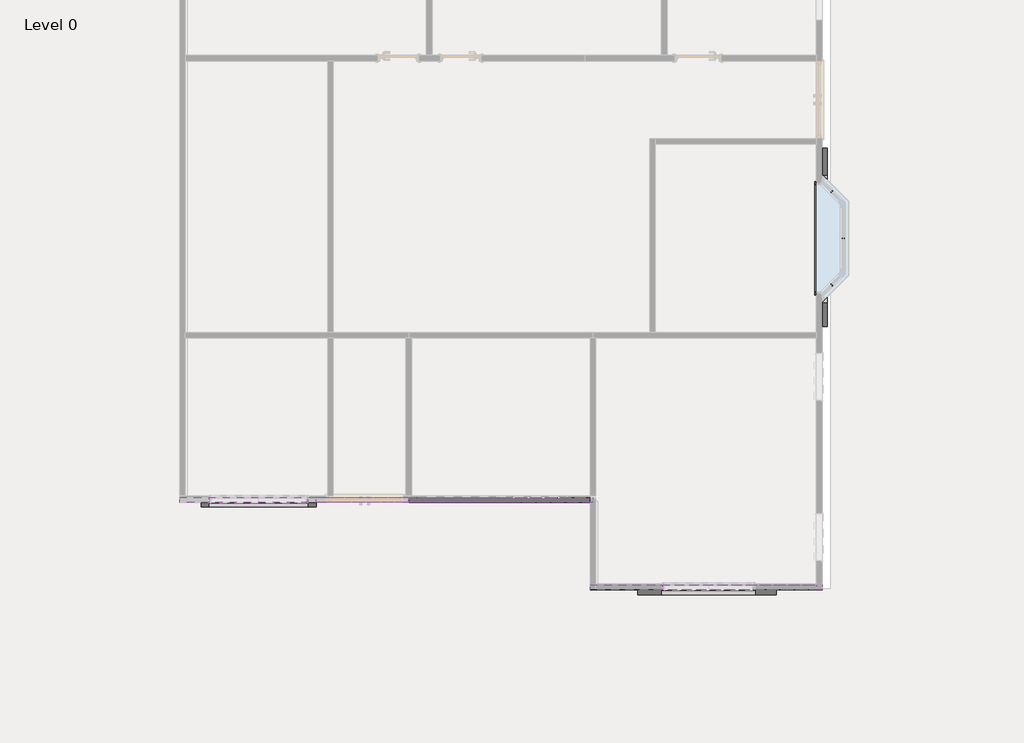
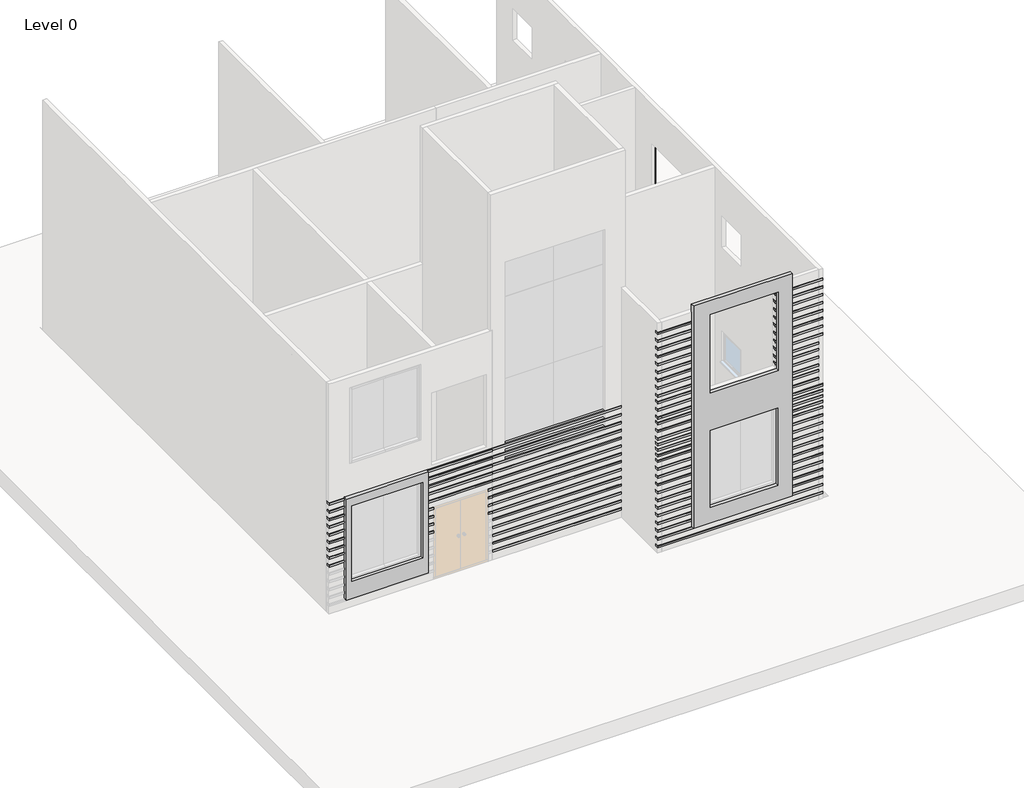
# One storey, part 5 of 5: 60 proxies.
"""IFC4 building model written with IfcOpenShell, lengths in millimetres."""

from ifc_helpers import new_model, si_unit, frame, origin, place, context, project, spatial, polyline, outline, extrude, transform, mapped, element, save
from components import generic_models_1_generic_models_1_954afae2, generic_models_4_generic_models_4_8888209d, generic_models_7_generic_models_7_fc47f9bb, muntin_pattern_2x2_muntin_pattern_2x2_511ed329, muntin_pattern_2x2_muntin_pattern_2x2_63bd3b25, trim_window_interior_flat_picture_frame_e25f2530

model = new_model("IFC4")

# Units and contexts
model_context = context("Model", 3, world=origin())
ifc_project = project(units=[si_unit("LENGTHUNIT", "METRE", prefix="MILLI")], contexts=[model_context])

# Site, building, storey
site = spatial("IfcSite", under=ifc_project)
building = spatial("IfcBuilding", under=site)
storey = spatial("IfcBuildingStorey", under=building, Name="Level 0", Elevation=0.0)

# Proxies
placement = place(None, origin())
element("IfcBuildingElementProxy", 1, Name="Cornice", ObjectType="Cornice", at=placement, inside=storey, context=model_context, shape_type="SweptSolid", body=[
    extrude(outline(polyline([(-2780.5468048, 1828.8), (-2883.0468048, 1828.8), (-2883.0468048, 1883.8), (-2863.0468048, 1903.8), (-2780.5468048, 1903.8), (-2780.5468048, 1828.8)])), frame((-14910.579089, 0.0, 0.0), z_axis=(1.0, 0.0, 0.0), x_axis=(0.0, 1.0, 0.0)), (0.0, 0.0, 1.0), 3562.35),
])
element("IfcBuildingElementProxy", 2, Name="Cornice", ObjectType="Cornice", at=placement, inside=storey, context=model_context, shape_type="SweptSolid", body=[
    extrude(outline(polyline([(-2780.5468048, 2057.4), (-2883.0468048, 2057.4), (-2883.0468048, 2112.4), (-2863.0468048, 2132.4), (-2780.5468048, 2132.4), (-2780.5468048, 2057.4)])), frame((-14910.579089, 0.0, 0.0), z_axis=(1.0, 0.0, 0.0), x_axis=(0.0, 1.0, 0.0)), (0.0, 0.0, 1.0), 3562.35),
])
element("IfcBuildingElementProxy", 3, Name="Cornice", ObjectType="Cornice", at=placement, inside=storey, context=model_context, shape_type="SweptSolid", body=[
    extrude(outline(polyline([(-2780.5468048, 2286.0), (-2883.0468048, 2286.0), (-2883.0468048, 2341.0), (-2863.0468048, 2361.0), (-2780.5468048, 2361.0), (-2780.5468048, 2286.0)])), frame((-16727.530247, 0.0, 0.0), z_axis=(1.0, 0.0, 0.0), x_axis=(0.0, 1.0, 0.0)), (0.0, 0.0, 1.0), 5379.301158),
])
element("IfcBuildingElementProxy", 4, Name="Cornice", ObjectType="Cornice", at=placement, inside=storey, context=model_context, shape_type="SweptSolid", body=[
    extrude(outline(polyline([(-2780.5468048, 2514.6), (-2883.0468048, 2514.6), (-2883.0468048, 2569.6), (-2863.0468048, 2589.6), (-2780.5468048, 2589.6), (-2780.5468048, 2514.6)])), frame((-16727.530247, 0.0, 0.0), z_axis=(1.0, 0.0, 0.0), x_axis=(0.0, 1.0, 0.0)), (0.0, 0.0, 1.0), 5379.301158),
])
element("IfcBuildingElementProxy", 5, Name="Cornice", ObjectType="Cornice", at=placement, inside=storey, context=model_context, shape_type="SweptSolid", body=[
    extrude(outline(polyline([(-2780.5468048, 1600.2), (-2883.0468048, 1600.2), (-2883.0468048, 1655.2), (-2863.0468048, 1675.2), (-2780.5468048, 1675.2), (-2780.5468048, 1600.2)])), frame((-14910.579089, 0.0, 0.0), z_axis=(1.0, 0.0, 0.0), x_axis=(0.0, 1.0, 0.0)), (0.0, 0.0, 1.0), 3562.35),
])
element("IfcBuildingElementProxy", 6, Name="Cornice", ObjectType="Cornice", at=placement, inside=storey, context=model_context, shape_type="SweptSolid", body=[
    extrude(outline(polyline([(-2780.5468048, 1371.6), (-2883.0468048, 1371.6), (-2883.0468048, 1426.6), (-2863.0468048, 1446.6), (-2780.5468048, 1446.6), (-2780.5468048, 1371.6)])), frame((-14910.579089, 0.0, 0.0), z_axis=(1.0, 0.0, 0.0), x_axis=(0.0, 1.0, 0.0)), (0.0, 0.0, 1.0), 3562.35),
])
element("IfcBuildingElementProxy", 7, Name="Cornice", ObjectType="Cornice", at=placement, inside=storey, context=model_context, shape_type="SweptSolid", body=[
    extrude(outline(polyline([(-2780.5468048, 1143.0), (-2883.0468048, 1143.0), (-2883.0468048, 1198.0), (-2863.0468048, 1218.0), (-2780.5468048, 1218.0), (-2780.5468048, 1143.0)])), frame((-14910.579089, 0.0, 0.0), z_axis=(1.0, 0.0, 0.0), x_axis=(0.0, 1.0, 0.0)), (0.0, 0.0, 1.0), 3562.35),
])
element("IfcBuildingElementProxy", 8, Name="Cornice", ObjectType="Cornice", at=placement, inside=storey, context=model_context, shape_type="SweptSolid", body=[
    extrude(outline(polyline([(-2780.5468048, 914.4), (-2883.0468048, 914.4), (-2883.0468048, 969.4), (-2863.0468048, 989.4), (-2780.5468048, 989.4), (-2780.5468048, 914.4)])), frame((-14910.579089, 0.0, 0.0), z_axis=(1.0, 0.0, 0.0), x_axis=(0.0, 1.0, 0.0)), (0.0, 0.0, 1.0), 3562.35),
])
element("IfcBuildingElementProxy", 9, Name="Cornice", ObjectType="Cornice", at=placement, inside=storey, context=model_context, shape_type="SweptSolid", body=[
    extrude(outline(polyline([(-2780.5468048, 685.8), (-2883.0468048, 685.8), (-2883.0468048, 740.8), (-2863.0468048, 760.8), (-2780.5468048, 760.8), (-2780.5468048, 685.8)])), frame((-14910.579089, 0.0, 0.0), z_axis=(1.0, 0.0, 0.0), x_axis=(0.0, 1.0, 0.0)), (0.0, 0.0, 1.0), 3562.35),
])
element("IfcBuildingElementProxy", 10, Name="Cornice", ObjectType="Cornice", at=placement, inside=storey, context=model_context, shape_type="SweptSolid", body=[
    extrude(outline(polyline([(-2780.5468048, 457.2), (-2883.0468048, 457.2), (-2883.0468048, 512.2), (-2863.0468048, 532.2), (-2780.5468048, 532.2), (-2780.5468048, 457.2)])), frame((-14910.579089, 0.0, 0.0), z_axis=(1.0, 0.0, 0.0), x_axis=(0.0, 1.0, 0.0)), (0.0, 0.0, 1.0), 3562.35),
])
element("IfcBuildingElementProxy", 11, Name="Cornice", ObjectType="Cornice", at=placement, inside=storey, context=model_context, shape_type="SweptSolid", body=[
    extrude(outline(polyline([(-2780.5468048, 228.6), (-2883.0468048, 228.6), (-2883.0468048, 283.6), (-2863.0468048, 303.6), (-2780.5468048, 303.6), (-2780.5468048, 228.6)])), frame((-14910.579089, 0.0, 0.0), z_axis=(1.0, 0.0, 0.0), x_axis=(0.0, 1.0, 0.0)), (0.0, 0.0, 1.0), 3562.35),
])
element("IfcBuildingElementProxy", 12, Name="Cornice", ObjectType="Cornice", at=placement, inside=storey, context=model_context, shape_type="SweptSolid", body=[
    extrude(outline(polyline([(-2780.5468048, 2743.2), (-2883.0468048, 2743.2), (-2883.0468048, 2798.2), (-2863.0468048, 2818.2), (-2780.5468048, 2818.2), (-2780.5468048, 2743.2)])), frame((-16727.530247, 0.0, 0.0), z_axis=(1.0, 0.0, 0.0), x_axis=(0.0, 1.0, 0.0)), (0.0, 0.0, 1.0), 5436.451158),
    extrude(outline(polyline([(-2780.5468048, 2743.2), (-2883.0468048, 2743.2), (-2883.0468048, 2798.2), (-2863.0468048, 2818.2), (-2780.5468048, 2818.2), (-2780.5468048, 2743.2)])), frame((-16727.530247, 0.0, 0.0), z_axis=(1.0, 0.0, 0.0), x_axis=(0.0, 1.0, 0.0)), (0.0, 0.0, 1.0), 5436.451158),
])
element("IfcBuildingElementProxy", 13, Name="Cornice", ObjectType="Cornice", at=placement, inside=storey, context=model_context, shape_type="SweptSolid", body=[
    extrude(outline(polyline([(-2780.5468048, 2971.8), (-2883.0468048, 2971.8), (-2883.0468048, 3026.8), (-2863.0468048, 3046.8), (-2780.5468048, 3046.8), (-2780.5468048, 2971.8)])), frame((-16727.530247, 0.0, 0.0), z_axis=(1.0, 0.0, 0.0), x_axis=(0.0, 1.0, 0.0)), (0.0, 0.0, 1.0), 5436.451158),
    extrude(outline(polyline([(-2780.5468048, 2971.8), (-2883.0468048, 2971.8), (-2883.0468048, 3026.8), (-2863.0468048, 3046.8), (-2780.5468048, 3046.8), (-2780.5468048, 2971.8)])), frame((-16727.530247, 0.0, 0.0), z_axis=(1.0, 0.0, 0.0), x_axis=(0.0, 1.0, 0.0)), (0.0, 0.0, 1.0), 5436.451158),
])
element("IfcBuildingElementProxy", 14, Name="Cornice", ObjectType="Cornice", at=placement, inside=storey, context=model_context, shape_type="SweptSolid", body=[
    extrude(outline(polyline([(-2780.5468048, 3200.4), (-2883.0468048, 3200.4), (-2883.0468048, 3255.4), (-2863.0468048, 3275.4), (-2780.5468048, 3275.4), (-2780.5468048, 3200.4)])), frame((-16727.530247, 0.0, 0.0), z_axis=(1.0, 0.0, 0.0), x_axis=(0.0, 1.0, 0.0)), (0.0, 0.0, 1.0), 5436.451158),
    extrude(outline(polyline([(-2780.5468048, 3200.4), (-2883.0468048, 3200.4), (-2883.0468048, 3255.4), (-2863.0468048, 3275.4), (-2780.5468048, 3275.4), (-2780.5468048, 3200.4)])), frame((-16727.530247, 0.0, 0.0), z_axis=(1.0, 0.0, 0.0), x_axis=(0.0, 1.0, 0.0)), (0.0, 0.0, 1.0), 5436.451158),
])
element("IfcBuildingElementProxy", 15, Name="Cornice", ObjectType="Cornice", at=placement, inside=storey, context=model_context, shape_type="SweptSolid", body=[
    extrude(outline(polyline([(-4501.3968048, 152.4), (-4603.8968048, 152.4), (-4603.8968048, 207.4), (-4583.8968048, 227.4), (-4501.3968048, 227.4), (-4501.3968048, 152.4)])), frame((-11348.229089, 0.0, 0.0), z_axis=(1.0, 0.0, 0.0), x_axis=(0.0, 1.0, 0.0)), (0.0, 0.0, 1.0), 4559.3),
])
element("IfcBuildingElementProxy", 16, Name="Cornice", ObjectType="Cornice", at=placement, inside=storey, context=model_context, shape_type="SweptSolid", body=[
    extrude(outline(polyline([(-4501.3968048, 381.0), (-4603.8968048, 381.0), (-4603.8968048, 436.0), (-4583.8968048, 456.0), (-4501.3968048, 456.0), (-4501.3968048, 381.0)])), frame((-11348.229089, 0.0, 0.0), z_axis=(1.0, 0.0, 0.0), x_axis=(0.0, 1.0, 0.0)), (0.0, 0.0, 1.0), 4559.3),
])
element("IfcBuildingElementProxy", 17, Name="Cornice", ObjectType="Cornice", at=placement, inside=storey, context=model_context, shape_type="SweptSolid", body=[
    extrude(outline(polyline([(-4501.3968048, 609.6), (-4603.8968048, 609.6), (-4603.8968048, 664.6), (-4583.8968048, 684.6), (-4501.3968048, 684.6), (-4501.3968048, 609.6)])), frame((-11348.229089, 0.0, 0.0), z_axis=(1.0, 0.0, 0.0), x_axis=(0.0, 1.0, 0.0)), (0.0, 0.0, 1.0), 4559.3),
])
element("IfcBuildingElementProxy", 18, Name="Cornice", ObjectType="Cornice", at=placement, inside=storey, context=model_context, shape_type="SweptSolid", body=[
    extrude(outline(polyline([(-4501.3968048, 830.4106439), (-4603.8968048, 830.4106439), (-4603.8968048, 885.4106439), (-4583.8968048, 905.4106439), (-4501.3968048, 905.4106439), (-4501.3968048, 830.4106439)])), frame((-11348.229089, 0.0, 0.0), z_axis=(1.0, 0.0, 0.0), x_axis=(0.0, 1.0, 0.0)), (0.0, 0.0, 1.0), 4559.3),
])
element("IfcBuildingElementProxy", 19, Name="Cornice", ObjectType="Cornice", at=placement, inside=storey, context=model_context, shape_type="SweptSolid", body=[
    extrude(outline(polyline([(-4501.3968048, 1059.0106439), (-4603.8968048, 1059.0106439), (-4603.8968048, 1114.0106439), (-4583.8968048, 1134.0106439), (-4501.3968048, 1134.0106439), (-4501.3968048, 1059.0106439)])), frame((-8102.129089, 0.0, 0.0), z_axis=(1.0, 0.0, 0.0), x_axis=(0.0, 1.0, 0.0)), (0.0, 0.0, 1.0), 1313.2),
    extrude(outline(polyline([(-4501.3968048, 1059.0106439), (-4603.8968048, 1059.0106439), (-4603.8968048, 1114.0106439), (-4583.8968048, 1134.0106439), (-4501.3968048, 1134.0106439), (-4501.3968048, 1059.0106439)])), frame((-11348.229089, 0.0, 0.0), z_axis=(1.0, 0.0, 0.0), x_axis=(0.0, 1.0, 0.0)), (0.0, 0.0, 1.0), 1417.3),
])
element("IfcBuildingElementProxy", 20, Name="Cornice", ObjectType="Cornice", at=placement, inside=storey, context=model_context, shape_type="SweptSolid", body=[
    extrude(outline(polyline([(-4501.3968048, 1279.8212878), (-4603.8968048, 1279.8212878), (-4603.8968048, 1334.8212878), (-4583.8968048, 1354.8212878), (-4501.3968048, 1354.8212878), (-4501.3968048, 1279.8212878)])), frame((-8102.129089, 0.0, 0.0), z_axis=(1.0, 0.0, 0.0), x_axis=(0.0, 1.0, 0.0)), (0.0, 0.0, 1.0), 1313.2),
    extrude(outline(polyline([(-4501.3968048, 1279.8212878), (-4603.8968048, 1279.8212878), (-4603.8968048, 1334.8212878), (-4583.8968048, 1354.8212878), (-4501.3968048, 1354.8212878), (-4501.3968048, 1279.8212878)])), frame((-11348.229089, 0.0, 0.0), z_axis=(1.0, 0.0, 0.0), x_axis=(0.0, 1.0, 0.0)), (0.0, 0.0, 1.0), 1417.3),
])
element("IfcBuildingElementProxy", 21, Name="Cornice", ObjectType="Cornice", at=placement, inside=storey, context=model_context, shape_type="SweptSolid", body=[
    extrude(outline(polyline([(-4501.3968048, 1500.6319317), (-4603.8968048, 1500.6319317), (-4603.8968048, 1555.6319317), (-4583.8968048, 1575.6319317), (-4501.3968048, 1575.6319317), (-4501.3968048, 1500.6319317)])), frame((-8102.129089, 0.0, 0.0), z_axis=(1.0, 0.0, 0.0), x_axis=(0.0, 1.0, 0.0)), (0.0, 0.0, 1.0), 1313.2),
    extrude(outline(polyline([(-4501.3968048, 1500.6319317), (-4603.8968048, 1500.6319317), (-4603.8968048, 1555.6319317), (-4583.8968048, 1575.6319317), (-4501.3968048, 1575.6319317), (-4501.3968048, 1500.6319317)])), frame((-11348.229089, 0.0, 0.0), z_axis=(1.0, 0.0, 0.0), x_axis=(0.0, 1.0, 0.0)), (0.0, 0.0, 1.0), 1417.3),
])
element("IfcBuildingElementProxy", 22, Name="Cornice", ObjectType="Cornice", at=placement, inside=storey, context=model_context, shape_type="SweptSolid", body=[
    extrude(outline(polyline([(-4501.3968048, 1729.2319317), (-4603.8968048, 1729.2319317), (-4603.8968048, 1784.2319317), (-4583.8968048, 1804.2319317), (-4501.3968048, 1804.2319317), (-4501.3968048, 1729.2319317)])), frame((-8102.129089, 0.0, 0.0), z_axis=(1.0, 0.0, 0.0), x_axis=(0.0, 1.0, 0.0)), (0.0, 0.0, 1.0), 1313.2),
    extrude(outline(polyline([(-4501.3968048, 1729.2319317), (-4603.8968048, 1729.2319317), (-4603.8968048, 1784.2319317), (-4583.8968048, 1804.2319317), (-4501.3968048, 1804.2319317), (-4501.3968048, 1729.2319317)])), frame((-11348.229089, 0.0, 0.0), z_axis=(1.0, 0.0, 0.0), x_axis=(0.0, 1.0, 0.0)), (0.0, 0.0, 1.0), 1417.3),
])
element("IfcBuildingElementProxy", 23, Name="Cornice", ObjectType="Cornice", at=placement, inside=storey, context=model_context, shape_type="SweptSolid", body=[
    extrude(outline(polyline([(-4501.3968048, 1957.8319317), (-4603.8968048, 1957.8319317), (-4603.8968048, 2012.8319317), (-4583.8968048, 2032.8319317), (-4501.3968048, 2032.8319317), (-4501.3968048, 1957.8319317)])), frame((-8102.129089, 0.0, 0.0), z_axis=(1.0, 0.0, 0.0), x_axis=(0.0, 1.0, 0.0)), (0.0, 0.0, 1.0), 1313.2),
    extrude(outline(polyline([(-4501.3968048, 1957.8319317), (-4603.8968048, 1957.8319317), (-4603.8968048, 2012.8319317), (-4583.8968048, 2032.8319317), (-4501.3968048, 2032.8319317), (-4501.3968048, 1957.8319317)])), frame((-11348.229089, 0.0, 0.0), z_axis=(1.0, 0.0, 0.0), x_axis=(0.0, 1.0, 0.0)), (0.0, 0.0, 1.0), 1417.3),
])
element("IfcBuildingElementProxy", 24, Name="Cornice", ObjectType="Cornice", at=placement, inside=storey, context=model_context, shape_type="SweptSolid", body=[
    extrude(outline(polyline([(-4501.3968048, 2186.4319317), (-4603.8968048, 2186.4319317), (-4603.8968048, 2241.4319317), (-4583.8968048, 2261.4319317), (-4501.3968048, 2261.4319317), (-4501.3968048, 2186.4319317)])), frame((-8102.129089, 0.0, 0.0), z_axis=(1.0, 0.0, 0.0), x_axis=(0.0, 1.0, 0.0)), (0.0, 0.0, 1.0), 1313.2),
    extrude(outline(polyline([(-4501.3968048, 2186.4319317), (-4603.8968048, 2186.4319317), (-4603.8968048, 2241.4319317), (-4583.8968048, 2261.4319317), (-4501.3968048, 2261.4319317), (-4501.3968048, 2186.4319317)])), frame((-11348.229089, 0.0, 0.0), z_axis=(1.0, 0.0, 0.0), x_axis=(0.0, 1.0, 0.0)), (0.0, 0.0, 1.0), 1417.3),
])
element("IfcBuildingElementProxy", 25, Name="Cornice", ObjectType="Cornice", at=placement, inside=storey, context=model_context, shape_type="SweptSolid", body=[
    extrude(outline(polyline([(-4501.3968048, 2415.0319317), (-4603.8968048, 2415.0319317), (-4603.8968048, 2470.0319317), (-4583.8968048, 2490.0319317), (-4501.3968048, 2490.0319317), (-4501.3968048, 2415.0319317)])), frame((-8102.129089, 0.0, 0.0), z_axis=(1.0, 0.0, 0.0), x_axis=(0.0, 1.0, 0.0)), (0.0, 0.0, 1.0), 1313.2),
    extrude(outline(polyline([(-4501.3968048, 2415.0319317), (-4603.8968048, 2415.0319317), (-4603.8968048, 2470.0319317), (-4583.8968048, 2490.0319317), (-4501.3968048, 2490.0319317), (-4501.3968048, 2415.0319317)])), frame((-11348.229089, 0.0, 0.0), z_axis=(1.0, 0.0, 0.0), x_axis=(0.0, 1.0, 0.0)), (0.0, 0.0, 1.0), 1417.3),
])
element("IfcBuildingElementProxy", 26, Name="Cornice", ObjectType="Cornice", at=placement, inside=storey, context=model_context, shape_type="SweptSolid", body=[
    extrude(outline(polyline([(-4501.3968048, 2643.6319317), (-4603.8968048, 2643.6319317), (-4603.8968048, 2698.6319317), (-4583.8968048, 2718.6319317), (-4501.3968048, 2718.6319317), (-4501.3968048, 2643.6319317)])), frame((-8102.129089, 0.0, 0.0), z_axis=(1.0, 0.0, 0.0), x_axis=(0.0, 1.0, 0.0)), (0.0, 0.0, 1.0), 1313.2),
    extrude(outline(polyline([(-4501.3968048, 2643.6319317), (-4603.8968048, 2643.6319317), (-4603.8968048, 2698.6319317), (-4583.8968048, 2718.6319317), (-4501.3968048, 2718.6319317), (-4501.3968048, 2643.6319317)])), frame((-11348.229089, 0.0, 0.0), z_axis=(1.0, 0.0, 0.0), x_axis=(0.0, 1.0, 0.0)), (0.0, 0.0, 1.0), 1417.3),
])
element("IfcBuildingElementProxy", 27, Name="Cornice", ObjectType="Cornice", at=placement, inside=storey, context=model_context, shape_type="SweptSolid", body=[
    extrude(outline(polyline([(-4501.3968048, 2805.2765418), (-4603.8968048, 2805.2765418), (-4603.8968048, 2860.2765418), (-4583.8968048, 2880.2765418), (-4501.3968048, 2880.2765418), (-4501.3968048, 2805.2765418)])), frame((-8102.129089, 0.0, 0.0), z_axis=(1.0, 0.0, 0.0), x_axis=(0.0, 1.0, 0.0)), (0.0, 0.0, 1.0), 1313.2),
    extrude(outline(polyline([(-4501.3968048, 2805.2765418), (-4603.8968048, 2805.2765418), (-4603.8968048, 2860.2765418), (-4583.8968048, 2880.2765418), (-4501.3968048, 2880.2765418), (-4501.3968048, 2805.2765418)])), frame((-11348.229089, 0.0, 0.0), z_axis=(1.0, 0.0, 0.0), x_axis=(0.0, 1.0, 0.0)), (0.0, 0.0, 1.0), 1417.3),
])
element("IfcBuildingElementProxy", 28, Name="Cornice", ObjectType="Cornice", at=placement, inside=storey, context=model_context, shape_type="SweptSolid", body=[
    extrude(outline(polyline([(-4501.3968048, 2966.921152), (-4603.8968048, 2966.921152), (-4603.8968048, 3021.921152), (-4583.8968048, 3041.921152), (-4501.3968048, 3041.921152), (-4501.3968048, 2966.921152)])), frame((-8102.129089, 0.0, 0.0), z_axis=(1.0, 0.0, 0.0), x_axis=(0.0, 1.0, 0.0)), (0.0, 0.0, 1.0), 1313.2),
    extrude(outline(polyline([(-4501.3968048, 2966.921152), (-4603.8968048, 2966.921152), (-4603.8968048, 3021.921152), (-4583.8968048, 3041.921152), (-4501.3968048, 3041.921152), (-4501.3968048, 2966.921152)])), frame((-11348.229089, 0.0, 0.0), z_axis=(1.0, 0.0, 0.0), x_axis=(0.0, 1.0, 0.0)), (0.0, 0.0, 1.0), 1417.3),
])
element("IfcBuildingElementProxy", 29, Name="Cornice", ObjectType="Cornice", at=placement, inside=storey, context=model_context, shape_type="SweptSolid", body=[
    extrude(outline(polyline([(-4501.3968048, 3128.5657622), (-4603.8968048, 3128.5657622), (-4603.8968048, 3183.5657622), (-4583.8968048, 3203.5657622), (-4501.3968048, 3203.5657622), (-4501.3968048, 3128.5657622)])), frame((-8102.129089, 0.0, 0.0), z_axis=(1.0, 0.0, 0.0), x_axis=(0.0, 1.0, 0.0)), (0.0, 0.0, 1.0), 1313.2),
    extrude(outline(polyline([(-4501.3968048, 3128.5657622), (-4603.8968048, 3128.5657622), (-4603.8968048, 3183.5657622), (-4583.8968048, 3203.5657622), (-4501.3968048, 3203.5657622), (-4501.3968048, 3128.5657622)])), frame((-11348.229089, 0.0, 0.0), z_axis=(1.0, 0.0, 0.0), x_axis=(0.0, 1.0, 0.0)), (0.0, 0.0, 1.0), 1417.3),
])
element("IfcBuildingElementProxy", 30, Name="Cornice", ObjectType="Cornice", at=placement, inside=storey, context=model_context, shape_type="SweptSolid", body=[
    extrude(outline(polyline([(-2780.5468048, 1371.6), (-2883.0468048, 1371.6), (-2883.0468048, 1426.6), (-2863.0468048, 1446.6), (-2780.5468048, 1446.6), (-2780.5468048, 1371.6)])), frame((-15018.529089, 0.0, 0.0), z_axis=(1.0, 0.0, 0.0), x_axis=(0.0, 1.0, 0.0)), (0.0, 0.0, 1.0), 107.95),
    extrude(outline(polyline([(-2780.5468048, 1371.6), (-2883.0468048, 1371.6), (-2883.0468048, 1426.6), (-2863.0468048, 1446.6), (-2780.5468048, 1446.6), (-2780.5468048, 1371.6)])), frame((-16885.429089, 0.0, 0.0), z_axis=(1.0, 0.0, 0.0), x_axis=(0.0, 1.0, 0.0)), (0.0, 0.0, 1.0), 356.9),
    extrude(outline(polyline([(-2780.5468048, 1371.6), (-2883.0468048, 1371.6), (-2883.0468048, 1426.6), (-2863.0468048, 1446.6), (-2780.5468048, 1446.6), (-2780.5468048, 1371.6)])), frame((-19412.729089, 0.0, 0.0), z_axis=(1.0, 0.0, 0.0), x_axis=(0.0, 1.0, 0.0)), (0.0, 0.0, 1.0), 571.5),
])
element("IfcBuildingElementProxy", 31, Name="Cornice", ObjectType="Cornice", at=placement, inside=storey, context=model_context, shape_type="SweptSolid", body=[
    extrude(outline(polyline([(-2780.5468048, 1600.2), (-2883.0468048, 1600.2), (-2883.0468048, 1655.2), (-2863.0468048, 1675.2), (-2780.5468048, 1675.2), (-2780.5468048, 1600.2)])), frame((-15018.529089, 0.0, 0.0), z_axis=(1.0, 0.0, 0.0), x_axis=(0.0, 1.0, 0.0)), (0.0, 0.0, 1.0), 107.95),
    extrude(outline(polyline([(-2780.5468048, 1600.2), (-2883.0468048, 1600.2), (-2883.0468048, 1655.2), (-2863.0468048, 1675.2), (-2780.5468048, 1675.2), (-2780.5468048, 1600.2)])), frame((-16885.429089, 0.0, 0.0), z_axis=(1.0, 0.0, 0.0), x_axis=(0.0, 1.0, 0.0)), (0.0, 0.0, 1.0), 356.9),
    extrude(outline(polyline([(-2780.5468048, 1600.2), (-2883.0468048, 1600.2), (-2883.0468048, 1655.2), (-2863.0468048, 1675.2), (-2780.5468048, 1675.2), (-2780.5468048, 1600.2)])), frame((-19412.729089, 0.0, 0.0), z_axis=(1.0, 0.0, 0.0), x_axis=(0.0, 1.0, 0.0)), (0.0, 0.0, 1.0), 571.5),
])
element("IfcBuildingElementProxy", 32, Name="Cornice", ObjectType="Cornice", at=placement, inside=storey, context=model_context, shape_type="SweptSolid", body=[
    extrude(outline(polyline([(-2780.5468048, 1821.0106439), (-2883.0468048, 1821.0106439), (-2883.0468048, 1876.0106439), (-2863.0468048, 1896.0106439), (-2780.5468048, 1896.0106439), (-2780.5468048, 1821.0106439)])), frame((-15018.529089, 0.0, 0.0), z_axis=(1.0, 0.0, 0.0), x_axis=(0.0, 1.0, 0.0)), (0.0, 0.0, 1.0), 107.95),
    extrude(outline(polyline([(-2780.5468048, 1821.0106439), (-2883.0468048, 1821.0106439), (-2883.0468048, 1876.0106439), (-2863.0468048, 1896.0106439), (-2780.5468048, 1896.0106439), (-2780.5468048, 1821.0106439)])), frame((-16885.429089, 0.0, 0.0), z_axis=(1.0, 0.0, 0.0), x_axis=(0.0, 1.0, 0.0)), (0.0, 0.0, 1.0), 356.9),
    extrude(outline(polyline([(-2780.5468048, 1821.0106439), (-2883.0468048, 1821.0106439), (-2883.0468048, 1876.0106439), (-2863.0468048, 1896.0106439), (-2780.5468048, 1896.0106439), (-2780.5468048, 1821.0106439)])), frame((-19412.729089, 0.0, 0.0), z_axis=(1.0, 0.0, 0.0), x_axis=(0.0, 1.0, 0.0)), (0.0, 0.0, 1.0), 571.5),
])
element("IfcBuildingElementProxy", 33, Name="Cornice", ObjectType="Cornice", at=placement, inside=storey, context=model_context, shape_type="SweptSolid", body=[
    extrude(outline(polyline([(-2780.5468048, 2049.6106439), (-2883.0468048, 2049.6106439), (-2883.0468048, 2104.6106439), (-2863.0468048, 2124.6106439), (-2780.5468048, 2124.6106439), (-2780.5468048, 2049.6106439)])), frame((-15018.529089, 0.0, 0.0), z_axis=(1.0, 0.0, 0.0), x_axis=(0.0, 1.0, 0.0)), (0.0, 0.0, 1.0), 107.95),
    extrude(outline(polyline([(-2780.5468048, 2049.6106439), (-2883.0468048, 2049.6106439), (-2883.0468048, 2104.6106439), (-2863.0468048, 2124.6106439), (-2780.5468048, 2124.6106439), (-2780.5468048, 2049.6106439)])), frame((-16885.429089, 0.0, 0.0), z_axis=(1.0, 0.0, 0.0), x_axis=(0.0, 1.0, 0.0)), (0.0, 0.0, 1.0), 356.9),
    extrude(outline(polyline([(-2780.5468048, 2049.6106439), (-2883.0468048, 2049.6106439), (-2883.0468048, 2104.6106439), (-2863.0468048, 2124.6106439), (-2780.5468048, 2124.6106439), (-2780.5468048, 2049.6106439)])), frame((-19412.729089, 0.0, 0.0), z_axis=(1.0, 0.0, 0.0), x_axis=(0.0, 1.0, 0.0)), (0.0, 0.0, 1.0), 571.5),
])
element("IfcBuildingElementProxy", 34, Name="Cornice", ObjectType="Cornice", at=placement, inside=storey, context=model_context, shape_type="SweptSolid", body=[
    extrude(outline(polyline([(-2780.5468048, 2278.2106439), (-2883.0468048, 2278.2106439), (-2883.0468048, 2333.2106439), (-2863.0468048, 2353.2106439), (-2780.5468048, 2353.2106439), (-2780.5468048, 2278.2106439)])), frame((-16885.429089, 0.0, 0.0), z_axis=(1.0, 0.0, 0.0), x_axis=(0.0, 1.0, 0.0)), (0.0, 0.0, 1.0), 1974.85),
    extrude(outline(polyline([(-2780.5468048, 2278.2106439), (-2883.0468048, 2278.2106439), (-2883.0468048, 2333.2106439), (-2863.0468048, 2353.2106439), (-2780.5468048, 2353.2106439), (-2780.5468048, 2278.2106439)])), frame((-19412.729089, 0.0, 0.0), z_axis=(1.0, 0.0, 0.0), x_axis=(0.0, 1.0, 0.0)), (0.0, 0.0, 1.0), 571.5),
])
element("IfcBuildingElementProxy", 35, Name="Cornice", ObjectType="Cornice", at=placement, inside=storey, context=model_context, shape_type="SweptSolid", body=[
    extrude(outline(polyline([(-2780.5468048, 2506.8106439), (-2883.0468048, 2506.8106439), (-2883.0468048, 2561.8106439), (-2863.0468048, 2581.8106439), (-2780.5468048, 2581.8106439), (-2780.5468048, 2506.8106439)])), frame((-16885.429089, 0.0, 0.0), z_axis=(1.0, 0.0, 0.0), x_axis=(0.0, 1.0, 0.0)), (0.0, 0.0, 1.0), 1974.85),
    extrude(outline(polyline([(-2780.5468048, 2506.8106439), (-2883.0468048, 2506.8106439), (-2883.0468048, 2561.8106439), (-2863.0468048, 2581.8106439), (-2780.5468048, 2581.8106439), (-2780.5468048, 2506.8106439)])), frame((-19412.729089, 0.0, 0.0), z_axis=(1.0, 0.0, 0.0), x_axis=(0.0, 1.0, 0.0)), (0.0, 0.0, 1.0), 571.5),
])
element("IfcBuildingElementProxy", 36, Name="Cornice", ObjectType="Cornice", at=placement, inside=storey, context=model_context, shape_type="SweptSolid", body=[
    extrude(outline(polyline([(-2780.5468048, 2720.4284072), (-2883.0468048, 2720.4284072), (-2883.0468048, 2775.4284072), (-2863.0468048, 2795.4284072), (-2780.5468048, 2795.4284072), (-2780.5468048, 2720.4284072)])), frame((-16885.429089, 0.0, 0.0), z_axis=(1.0, 0.0, 0.0), x_axis=(0.0, 1.0, 0.0)), (0.0, 0.0, 1.0), 1974.85),
    extrude(outline(polyline([(-2780.5468048, 2720.4284072), (-2883.0468048, 2720.4284072), (-2883.0468048, 2775.4284072), (-2863.0468048, 2795.4284072), (-2780.5468048, 2795.4284072), (-2780.5468048, 2720.4284072)])), frame((-19412.729089, 0.0, 0.0), z_axis=(1.0, 0.0, 0.0), x_axis=(0.0, 1.0, 0.0)), (0.0, 0.0, 1.0), 571.5),
])
element("IfcBuildingElementProxy", 37, Name="Cornice", ObjectType="Cornice", at=placement, inside=storey, context=model_context, shape_type="SweptSolid", body=[
    extrude(outline(polyline([(-2780.5468048, 2949.0284072), (-2883.0468048, 2949.0284072), (-2883.0468048, 3004.0284072), (-2863.0468048, 3024.0284072), (-2780.5468048, 3024.0284072), (-2780.5468048, 2949.0284072)])), frame((-16885.429089, 0.0, 0.0), z_axis=(1.0, 0.0, 0.0), x_axis=(0.0, 1.0, 0.0)), (0.0, 0.0, 1.0), 1974.85),
    extrude(outline(polyline([(-2780.5468048, 2949.0284072), (-2883.0468048, 2949.0284072), (-2883.0468048, 3004.0284072), (-2863.0468048, 3024.0284072), (-2780.5468048, 3024.0284072), (-2780.5468048, 2949.0284072)])), frame((-19412.729089, 0.0, 0.0), z_axis=(1.0, 0.0, 0.0), x_axis=(0.0, 1.0, 0.0)), (0.0, 0.0, 1.0), 571.5),
])
element("IfcBuildingElementProxy", 38, Name="Cornice", ObjectType="Cornice", at=placement, inside=storey, context=model_context, shape_type="SweptSolid", body=[
    extrude(outline(polyline([(-2780.5468048, 3177.6284072), (-2883.0468048, 3177.6284072), (-2883.0468048, 3232.6284072), (-2863.0468048, 3252.6284072), (-2780.5468048, 3252.6284072), (-2780.5468048, 3177.6284072)])), frame((-19412.729089, 0.0, 0.0), z_axis=(1.0, 0.0, 0.0), x_axis=(0.0, 1.0, 0.0)), (0.0, 0.0, 1.0), 4502.15),
])
element("IfcBuildingElementProxy", 39, Name="Cornice", ObjectType="Cornice", at=placement, inside=storey, context=model_context, shape_type="SweptSolid", body=[
    extrude(outline(polyline([(-4501.3968048, 3290.2103724), (-4603.8968048, 3290.2103724), (-4603.8968048, 3345.2103724), (-4583.8968048, 3365.2103724), (-4501.3968048, 3365.2103724), (-4501.3968048, 3290.2103724)])), frame((-11348.229089, 0.0, 0.0), z_axis=(1.0, 0.0, 0.0), x_axis=(0.0, 1.0, 0.0)), (0.0, 0.0, 1.0), 4559.3),
])
element("IfcBuildingElementProxy", 40, Name="Cornice", ObjectType="Cornice", at=placement, inside=storey, context=model_context, shape_type="SweptSolid", body=[
    extrude(outline(polyline([(-4501.3968048, 3518.8103724), (-4603.8968048, 3518.8103724), (-4603.8968048, 3573.8103724), (-4583.8968048, 3593.8103724), (-4501.3968048, 3593.8103724), (-4501.3968048, 3518.8103724)])), frame((-11348.229089, 0.0, 0.0), z_axis=(1.0, 0.0, 0.0), x_axis=(0.0, 1.0, 0.0)), (0.0, 0.0, 1.0), 4445.0),
])
element("IfcBuildingElementProxy", 41, Name="Cornice", ObjectType="Cornice", at=placement, inside=storey, context=model_context, shape_type="SweptSolid", body=[
    extrude(outline(polyline([(-4501.3968048, 3747.4103724), (-4603.8968048, 3747.4103724), (-4603.8968048, 3802.4103724), (-4583.8968048, 3822.4103724), (-4501.3968048, 3822.4103724), (-4501.3968048, 3747.4103724)])), frame((-11348.229089, 0.0, 0.0), z_axis=(1.0, 0.0, 0.0), x_axis=(0.0, 1.0, 0.0)), (0.0, 0.0, 1.0), 4445.0),
])
element("IfcBuildingElementProxy", 42, Name="Cornice", ObjectType="Cornice", at=placement, inside=storey, context=model_context, shape_type="SweptSolid", body=[
    extrude(outline(polyline([(-4501.3968048, 3909.0549826), (-4603.8968048, 3909.0549826), (-4603.8968048, 3964.0549826), (-4583.8968048, 3984.0549826), (-4501.3968048, 3984.0549826), (-4501.3968048, 3909.0549826)])), frame((-11348.229089, 0.0, 0.0), z_axis=(1.0, 0.0, 0.0), x_axis=(0.0, 1.0, 0.0)), (0.0, 0.0, 1.0), 4445.0),
])
element("IfcBuildingElementProxy", 43, Name="Cornice", ObjectType="Cornice", at=placement, inside=storey, context=model_context, shape_type="SweptSolid", body=[
    extrude(outline(polyline([(-4501.3968048, 4137.6549826), (-4603.8968048, 4137.6549826), (-4603.8968048, 4192.6549826), (-4583.8968048, 4212.6549826), (-4501.3968048, 4212.6549826), (-4501.3968048, 4137.6549826)])), frame((-11348.229089, 0.0, 0.0), z_axis=(1.0, 0.0, 0.0), x_axis=(0.0, 1.0, 0.0)), (0.0, 0.0, 1.0), 4445.0),
])
element("IfcBuildingElementProxy", 44, Name="Cornice", ObjectType="Cornice", at=placement, inside=storey, context=model_context, shape_type="SweptSolid", body=[
    extrude(outline(polyline([(-4501.3968048, 4358.4656265), (-4603.8968048, 4358.4656265), (-4603.8968048, 4413.4656265), (-4583.8968048, 4433.4656265), (-4501.3968048, 4433.4656265), (-4501.3968048, 4358.4656265)])), frame((-8102.129089, 0.0, 0.0), z_axis=(1.0, 0.0, 0.0), x_axis=(0.0, 1.0, 0.0)), (0.0, 0.0, 1.0), 1198.9),
    extrude(outline(polyline([(-4501.3968048, 4358.4656265), (-4603.8968048, 4358.4656265), (-4603.8968048, 4413.4656265), (-4583.8968048, 4433.4656265), (-4501.3968048, 4433.4656265), (-4501.3968048, 4358.4656265)])), frame((-11348.229089, 0.0, 0.0), z_axis=(1.0, 0.0, 0.0), x_axis=(0.0, 1.0, 0.0)), (0.0, 0.0, 1.0), 1417.3),
])
element("IfcBuildingElementProxy", 45, Name="Cornice", ObjectType="Cornice", at=placement, inside=storey, context=model_context, shape_type="SweptSolid", body=[
    extrude(outline(polyline([(-4501.3968048, 4545.5846362), (-4603.8968048, 4545.5846362), (-4603.8968048, 4600.5846362), (-4583.8968048, 4620.5846362), (-4501.3968048, 4620.5846362), (-4501.3968048, 4545.5846362)])), frame((-8102.129089, 0.0, 0.0), z_axis=(1.0, 0.0, 0.0), x_axis=(0.0, 1.0, 0.0)), (0.0, 0.0, 1.0), 1198.9),
    extrude(outline(polyline([(-4501.3968048, 4545.5846362), (-4603.8968048, 4545.5846362), (-4603.8968048, 4600.5846362), (-4583.8968048, 4620.5846362), (-4501.3968048, 4620.5846362), (-4501.3968048, 4545.5846362)])), frame((-11348.229089, 0.0, 0.0), z_axis=(1.0, 0.0, 0.0), x_axis=(0.0, 1.0, 0.0)), (0.0, 0.0, 1.0), 1417.3),
])
element("IfcBuildingElementProxy", 46, Name="Cornice", ObjectType="Cornice", at=placement, inside=storey, context=model_context, shape_type="SweptSolid", body=[
    extrude(outline(polyline([(-4501.3968048, 4774.1846362), (-4603.8968048, 4774.1846362), (-4603.8968048, 4829.1846362), (-4583.8968048, 4849.1846362), (-4501.3968048, 4849.1846362), (-4501.3968048, 4774.1846362)])), frame((-8102.129089, 0.0, 0.0), z_axis=(1.0, 0.0, 0.0), x_axis=(0.0, 1.0, 0.0)), (0.0, 0.0, 1.0), 1313.2),
    extrude(outline(polyline([(-4501.3968048, 4774.1846362), (-4603.8968048, 4774.1846362), (-4603.8968048, 4829.1846362), (-4583.8968048, 4849.1846362), (-4501.3968048, 4849.1846362), (-4501.3968048, 4774.1846362)])), frame((-11348.229089, 0.0, 0.0), z_axis=(1.0, 0.0, 0.0), x_axis=(0.0, 1.0, 0.0)), (0.0, 0.0, 1.0), 1417.3),
])
element("IfcBuildingElementProxy", 47, Name="Cornice", ObjectType="Cornice", at=placement, inside=storey, context=model_context, shape_type="SweptSolid", body=[
    extrude(outline(polyline([(-4501.3968048, 5002.7846362), (-4603.8968048, 5002.7846362), (-4603.8968048, 5057.7846362), (-4583.8968048, 5077.7846362), (-4501.3968048, 5077.7846362), (-4501.3968048, 5002.7846362)])), frame((-8102.129089, 0.0, 0.0), z_axis=(1.0, 0.0, 0.0), x_axis=(0.0, 1.0, 0.0)), (0.0, 0.0, 1.0), 1313.2),
    extrude(outline(polyline([(-4501.3968048, 5002.7846362), (-4603.8968048, 5002.7846362), (-4603.8968048, 5057.7846362), (-4583.8968048, 5077.7846362), (-4501.3968048, 5077.7846362), (-4501.3968048, 5002.7846362)])), frame((-11348.229089, 0.0, 0.0), z_axis=(1.0, 0.0, 0.0), x_axis=(0.0, 1.0, 0.0)), (0.0, 0.0, 1.0), 1417.3),
])
element("IfcBuildingElementProxy", 48, Name="Cornice", ObjectType="Cornice", at=placement, inside=storey, context=model_context, shape_type="SweptSolid", body=[
    extrude(outline(polyline([(-4501.3968048, 5231.3846362), (-4603.8968048, 5231.3846362), (-4603.8968048, 5286.3846362), (-4583.8968048, 5306.3846362), (-4501.3968048, 5306.3846362), (-4501.3968048, 5231.3846362)])), frame((-8102.129089, 0.0, 0.0), z_axis=(1.0, 0.0, 0.0), x_axis=(0.0, 1.0, 0.0)), (0.0, 0.0, 1.0), 1313.2),
    extrude(outline(polyline([(-4501.3968048, 5231.3846362), (-4603.8968048, 5231.3846362), (-4603.8968048, 5286.3846362), (-4583.8968048, 5306.3846362), (-4501.3968048, 5306.3846362), (-4501.3968048, 5231.3846362)])), frame((-11348.229089, 0.0, 0.0), z_axis=(1.0, 0.0, 0.0), x_axis=(0.0, 1.0, 0.0)), (0.0, 0.0, 1.0), 1417.3),
])
element("IfcBuildingElementProxy", 49, Name="Cornice", ObjectType="Cornice", at=placement, inside=storey, context=model_context, shape_type="SweptSolid", body=[
    extrude(outline(polyline([(-4501.3968048, 5459.9846362), (-4603.8968048, 5459.9846362), (-4603.8968048, 5514.9846362), (-4583.8968048, 5534.9846362), (-4501.3968048, 5534.9846362), (-4501.3968048, 5459.9846362)])), frame((-8102.129089, 0.0, 0.0), z_axis=(1.0, 0.0, 0.0), x_axis=(0.0, 1.0, 0.0)), (0.0, 0.0, 1.0), 1313.2),
    extrude(outline(polyline([(-4501.3968048, 5459.9846362), (-4603.8968048, 5459.9846362), (-4603.8968048, 5514.9846362), (-4583.8968048, 5534.9846362), (-4501.3968048, 5534.9846362), (-4501.3968048, 5459.9846362)])), frame((-11348.229089, 0.0, 0.0), z_axis=(1.0, 0.0, 0.0), x_axis=(0.0, 1.0, 0.0)), (0.0, 0.0, 1.0), 1417.3),
])
element("IfcBuildingElementProxy", 50, Name="Cornice", ObjectType="Cornice", at=placement, inside=storey, context=model_context, shape_type="SweptSolid", body=[
    extrude(outline(polyline([(-4501.3968048, 5688.5846362), (-4603.8968048, 5688.5846362), (-4603.8968048, 5743.5846362), (-4583.8968048, 5763.5846362), (-4501.3968048, 5763.5846362), (-4501.3968048, 5688.5846362)])), frame((-8102.129089, 0.0, 0.0), z_axis=(1.0, 0.0, 0.0), x_axis=(0.0, 1.0, 0.0)), (0.0, 0.0, 1.0), 1313.2),
    extrude(outline(polyline([(-4501.3968048, 5688.5846362), (-4603.8968048, 5688.5846362), (-4603.8968048, 5743.5846362), (-4583.8968048, 5763.5846362), (-4501.3968048, 5763.5846362), (-4501.3968048, 5688.5846362)])), frame((-11348.229089, 0.0, 0.0), z_axis=(1.0, 0.0, 0.0), x_axis=(0.0, 1.0, 0.0)), (0.0, 0.0, 1.0), 1417.3),
])
element("IfcBuildingElementProxy", 51, Name="Cornice", ObjectType="Cornice", at=placement, inside=storey, context=model_context, shape_type="SweptSolid", body=[
    extrude(outline(polyline([(-4501.3968048, 5917.1846362), (-4603.8968048, 5917.1846362), (-4603.8968048, 5972.1846362), (-4583.8968048, 5992.1846362), (-4501.3968048, 5992.1846362), (-4501.3968048, 5917.1846362)])), frame((-8102.129089, 0.0, 0.0), z_axis=(1.0, 0.0, 0.0), x_axis=(0.0, 1.0, 0.0)), (0.0, 0.0, 1.0), 1313.2),
    extrude(outline(polyline([(-4501.3968048, 5917.1846362), (-4603.8968048, 5917.1846362), (-4603.8968048, 5972.1846362), (-4583.8968048, 5992.1846362), (-4501.3968048, 5992.1846362), (-4501.3968048, 5917.1846362)])), frame((-11348.229089, 0.0, 0.0), z_axis=(1.0, 0.0, 0.0), x_axis=(0.0, 1.0, 0.0)), (0.0, 0.0, 1.0), 1417.3),
])
element("IfcBuildingElementProxy", 52, Name="Cornice", ObjectType="Cornice", at=placement, inside=storey, context=model_context, shape_type="SweptSolid", body=[
    extrude(outline(polyline([(-4501.3968048, 6145.7846362), (-4603.8968048, 6145.7846362), (-4603.8968048, 6200.7846362), (-4583.8968048, 6220.7846362), (-4501.3968048, 6220.7846362), (-4501.3968048, 6145.7846362)])), frame((-8102.129089, 0.0, 0.0), z_axis=(1.0, 0.0, 0.0), x_axis=(0.0, 1.0, 0.0)), (0.0, 0.0, 1.0), 1313.2),
    extrude(outline(polyline([(-4501.3968048, 6145.7846362), (-4603.8968048, 6145.7846362), (-4603.8968048, 6200.7846362), (-4583.8968048, 6220.7846362), (-4501.3968048, 6220.7846362), (-4501.3968048, 6145.7846362)])), frame((-11348.229089, 0.0, 0.0), z_axis=(1.0, 0.0, 0.0), x_axis=(0.0, 1.0, 0.0)), (0.0, 0.0, 1.0), 1417.3),
])
element("IfcBuildingElementProxy", 53, Name="Cornice", ObjectType="Cornice", at=placement, inside=storey, context=model_context, shape_type="SweptSolid", body=[
    extrude(outline(polyline([(-4501.3968048, 6374.3846362), (-4603.8968048, 6374.3846362), (-4603.8968048, 6429.3846362), (-4583.8968048, 6449.3846362), (-4501.3968048, 6449.3846362), (-4501.3968048, 6374.3846362)])), frame((-8102.129089, 0.0, 0.0), z_axis=(1.0, 0.0, 0.0), x_axis=(0.0, 1.0, 0.0)), (0.0, 0.0, 1.0), 1313.2),
    extrude(outline(polyline([(-4501.3968048, 6374.3846362), (-4603.8968048, 6374.3846362), (-4603.8968048, 6429.3846362), (-4583.8968048, 6449.3846362), (-4501.3968048, 6449.3846362), (-4501.3968048, 6374.3846362)])), frame((-11348.229089, 0.0, 0.0), z_axis=(1.0, 0.0, 0.0), x_axis=(0.0, 1.0, 0.0)), (0.0, 0.0, 1.0), 1417.3),
])
generic_models_1_generic_models_1_shape = generic_models_1_generic_models_1_954afae2(model_context)
element("IfcBuildingElementProxy", 54, Name="Generic Models 1 : Generic Models 1", ObjectType="Generic Models 1 : Generic Models 1", at=placement, inside=storey, context=model_context, shape_type="MappedRepresentation", body=[
    mapped(generic_models_1_generic_models_1_shape, transform((0.0, 0.0, 0.0), x_axis=(1.0, 0.0, 0.0), y_axis=(0.0, 1.0, 0.0), z_axis=(0.0, 0.0, 1.0))),
])
generic_models_4_generic_models_4_shape = generic_models_4_generic_models_4_8888209d(model_context)
element("IfcBuildingElementProxy", 55, Name="Generic Models 4 : Generic Models 4", ObjectType="Generic Models 4 : Generic Models 4", at=placement, inside=storey, context=model_context, shape_type="MappedRepresentation", body=[
    mapped(generic_models_4_generic_models_4_shape, transform((0.0, 0.0, 0.0), x_axis=(1.0, 0.0, 0.0), y_axis=(0.0, 1.0, 0.0), z_axis=(0.0, 0.0, 1.0))),
])
generic_models_7_generic_models_7_shape = generic_models_7_generic_models_7_fc47f9bb(model_context)
element("IfcBuildingElementProxy", 56, Name="Generic Models 7 : Generic Models 7", ObjectType="Generic Models 7 : Generic Models 7", at=placement, inside=storey, context=model_context, shape_type="MappedRepresentation", body=[
    mapped(generic_models_7_generic_models_7_shape, transform((0.0, 0.0, 0.0), x_axis=(1.0, 0.0, 0.0), y_axis=(0.0, 1.0, 0.0), z_axis=(0.0, 0.0, 1.0))),
])
muntin_pattern_2x2_muntin_pattern_2x2_shape = muntin_pattern_2x2_muntin_pattern_2x2_511ed329(model_context)
element("IfcBuildingElementProxy", 57, Name="Muntin Pattern_2x2 : Muntin Pattern_2x2", ObjectType="Muntin Pattern_2x2 : Muntin Pattern_2x2", at=placement, inside=storey, context=model_context, shape_type="MappedRepresentation", body=[
    mapped(muntin_pattern_2x2_muntin_pattern_2x2_shape, transform((-6373.004089, 2308.5531952, 730.25), x_axis=(0.0, -1.0, 0.0), y_axis=(1.0, 0.0, 0.0), z_axis=(0.0, 0.0, 1.0))),
])
muntin_pattern_2x2_muntin_pattern_2x2_2_shape = muntin_pattern_2x2_muntin_pattern_2x2_63bd3b25(model_context)
element("IfcBuildingElementProxy", 58, Name="Muntin Pattern_2x2 : Muntin Pattern_2x2", ObjectType="Muntin Pattern_2x2 : Muntin Pattern_2x2", at=placement, inside=storey, context=model_context, shape_type="MappedRepresentation", body=[
    mapped(muntin_pattern_2x2_muntin_pattern_2x2_2_shape, transform((-6600.8997934, 3223.244924, 730.25), x_axis=(0.707106781186547, -0.7071067811865482, 0.0), y_axis=(0.7071067811865482, 0.707106781186547, 0.0), z_axis=(0.0, 0.0, 1.0))),
])
element("IfcBuildingElementProxy", 59, Name="Muntin Pattern_2x2 : Muntin Pattern_2x2", ObjectType="Muntin Pattern_2x2 : Muntin Pattern_2x2", at=placement, inside=storey, context=model_context, shape_type="MappedRepresentation", body=[
    mapped(muntin_pattern_2x2_muntin_pattern_2x2_2_shape, transform((-6600.8997934, 1393.8614664, 730.25), x_axis=(-0.7071067811865469, -0.7071067811865482, 0.0), y_axis=(0.7071067811865482, -0.7071067811865469, 0.0), z_axis=(0.0, 0.0, 1.0))),
])
trim_window_interior_flat_picture_frame_shape = trim_window_interior_flat_picture_frame_e25f2530(model_context)
element("IfcBuildingElementProxy", 60, Name="Trim-Window-Interior-Flat : Picture Frame", ObjectType="Trim-Window-Interior-Flat : Picture Frame", at=placement, inside=storey, context=model_context, shape_type="MappedRepresentation", body=[
    mapped(trim_window_interior_flat_picture_frame_shape, transform((-6903.229089, 2308.5531952, 2184.4), x_axis=(0.0, -1.0, 0.0), y_axis=(0.0, 0.0, 1.0), z_axis=(-1.0, 0.0, 0.0))),
])

save(model, "model.ifc")

# Revit data of these elements
# Type "Muntin Pattern_2x2 : Muntin Pattern_2x2"
#   Width [instance default] = 4' - 0"
#   Thickness = 0' - 0 1/2"
#   Height [instance default] = 4' - 0"
#   Distance = 0' - 0 3/4"
#   Interior Material [instance default] = none
#   Exterior Material [instance default] = none
#   Default Elevation = 0
# Type "Trim-Window-Interior-Flat : Picture Frame"
#   Trim Thickness_Picture Frame = 0' - 1 1/4"
#   Trim Width = 0' - 2 1/4"
#   Trim Thickness_with Sill = 0' - 0 3/4"
#   Sill Thickness = 0' - 1 1/4"
#   Opening Width [instance default] = 2' - 0"
#   Opening Height [instance default] = 3' - 0"
#   Default Elevation = 4' - 0"
#   Sill = no
#   Picture Frame = yes
#   Trim Material [instance default] = none
# Elements 1, 2, 3, 4, 5, 6, 7, 8, 9, 10, 11, 12, 13, 14, 15, 16, 17, 18, 19, 20, 21, 22, 23, 24, 25, 26, 27, 28, 29, 30, 31, 32, 33, 34, 35, 36, 37, 38, 39, 40, 41, 42, 43, 44, 45, 46, 47, 48, 49, 50, 51, 52, 53 (IfcBuildingElementProxy, "Cornice")
#   Phase Created = New Construction
#   Materials on its faces: "Default Wall"
# Element 54 (IfcBuildingElementProxy, "Generic Models 1 : Generic Models 1")
#   Phase Created = New Construction
# Element 55 (IfcBuildingElementProxy, "Generic Models 4 : Generic Models 4")
#   Phase Created = New Construction
# Element 56 (IfcBuildingElementProxy, "Generic Models 7 : Generic Models 7")
#   Phase Created = New Construction
#   Materials on its faces: "Wood Planks"
# Element 57 (IfcBuildingElementProxy, "Muntin Pattern_2x2 : Muntin Pattern_2x2")
#   Width = 3' - 8.88909"
#   Height = 4' - 6 1/2"
#   Interior Material = Wood - Stained
#   Exterior Material = Clad - White
#   Phase Created = New Construction
#   Materials on its faces: "Clad - White", "Wood - Stained"
# Elements 58, 59 (IfcBuildingElementProxy, "Muntin Pattern_2x2 : Muntin Pattern_2x2")
#   Width = 1' - 4.18808"
#   Height = 4' - 6 1/2"
#   Interior Material = Wood - Stained
#   Exterior Material = Clad - White
#   Phase Created = New Construction
#   Materials on its faces: "Clad - White", "Wood - Stained"
# Element 60 (IfcBuildingElementProxy, "Trim-Window-Interior-Flat : Picture Frame")
#   Opening Width = 7' - 0"
#   Opening Height = 5' - 2"
#   Trim Material = Wood - Stained
#   Phase Created = New Construction
#   Materials on its faces: "Wood - Stained"
# Materials
#   "Default Wall": colour RGB 128 128 128, transparency 0, Cost = 0
#   "Wood Planks": class "Wood", colour RGB 129 72 39, transparency 0, Description = "Physical material.", Cost = 0
#   "Clad - White": class "Wood", colour RGB 242 242 238, transparency 0, Cost = 0
#   "Wood - Stained": class "Wood", colour RGB 227 170 128, transparency 0, Cost = 0
